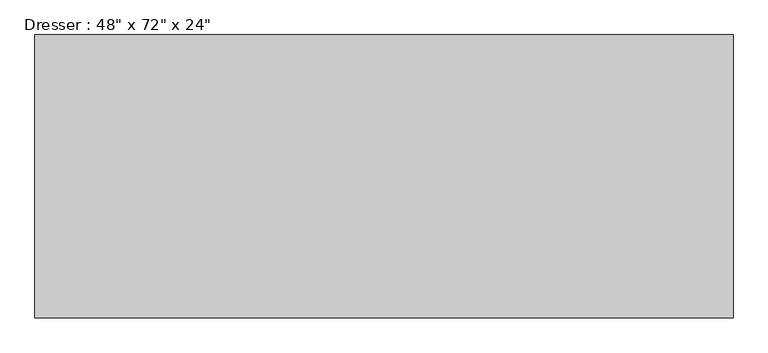
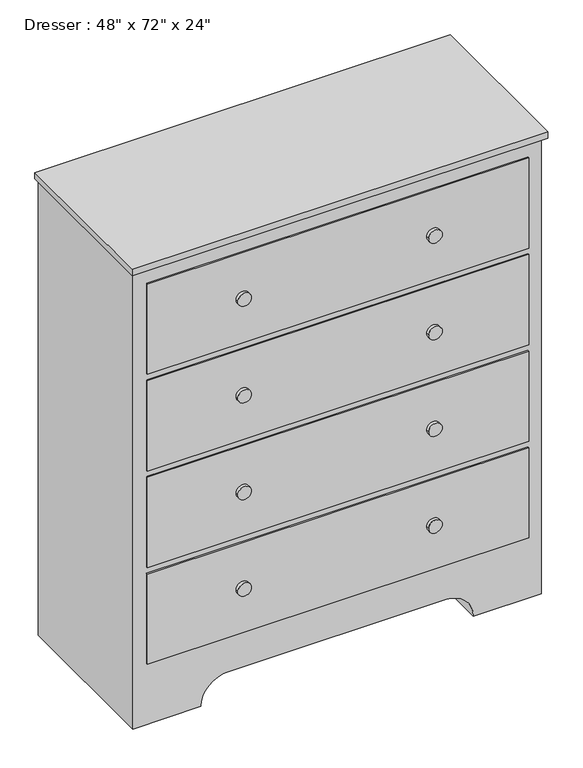
"""IFC4 building model written with IfcOpenShell, lengths in millimetres: furniture geometry."""

from ifc_helpers import new_model, si_unit, point, frame, frame_2d, origin, place, context, project, spatial, polyline, circle_curve, trimmed, segment, composite_curve, outline, extrude, source, transform, mapped, element, save


def furniture_d0678273(model_context):
    return source(origin(), model_context, "Body", "SweptSolid", [
        extrude(outline(polyline([(505.5067402, -58.3629541), (505.5067402, -687.0129541), (-1043.8932598, -687.0129541), (-1043.8932598, -58.3629541), (505.5067402, -58.3629541)])), frame((0.0, 0.0, 1803.4), z_axis=(0.0, 0.0, 1.0), x_axis=(1.0, 0.0, 0.0)), (0.0, 0.0, 1.0), 25.4),
        extrude(outline(composite_curve([segment(polyline([(0.0, 492.8067402), (1803.4, 492.8067402), (1803.4, -1031.1932598), (0.0, -1031.1932598), (0.0, -777.1932598)]), True, "CONTINUOUS"), segment(trimmed(circle_curve(frame_2d((0.0, -675.5932598)), 101.6), [point((0.0, -777.1932598))], [point((101.6, -675.5932598))], True, "CARTESIAN"), True, "CONTINUOUS"), segment(polyline([(101.6, -675.5932598), (101.6, 137.2067402)]), True, "CONTINUOUS"), segment(trimmed(circle_curve(frame_2d((0.0, 137.2067402)), 101.6), [point((101.6, 137.2067402))], [point((0.0, 238.8067402))], True, "CARTESIAN"), True, "CONTINUOUS"), segment(polyline([(0.0, 238.8067402), (0.0, 492.8067402)]), True, "CONTINUOUS")], self_intersect=False)), frame((0.0, -667.9629541, 0.0), z_axis=(0.0, 1.0, 0.0), x_axis=(0.0, 0.0, 1.0)), (0.0, 0.0, 1.0), 609.6),
        extrude(outline(composite_curve([segment(trimmed(circle_curve(frame_2d((1562.1, 86.4067402)), 25.4), [point((1562.1, 61.0067402))], [point((1562.1, 111.8067402))], False, "CARTESIAN"), True, "CONTINUOUS"), segment(trimmed(circle_curve(frame_2d((1562.1, 86.4067402)), 25.4), [point((1562.1, 111.8067402))], [point((1562.1, 61.0067402))], False, "CARTESIAN"), True, "CONTINUOUS")], self_intersect=False)), frame((0.0, -687.0129541, 0.0), z_axis=(0.0, 1.0, 0.0), x_axis=(0.0, 0.0, 1.0)), (0.0, 0.0, 1.0), 12.7),
        extrude(outline(composite_curve([segment(trimmed(circle_curve(frame_2d((1181.1, 86.4067402)), 25.4), [point((1181.1, 61.0067402))], [point((1181.1, 111.8067402))], False, "CARTESIAN"), True, "CONTINUOUS"), segment(trimmed(circle_curve(frame_2d((1181.1, 86.4067402)), 25.4), [point((1181.1, 111.8067402))], [point((1181.1, 61.0067402))], False, "CARTESIAN"), True, "CONTINUOUS")], self_intersect=False)), frame((0.0, -687.0129541, 0.0), z_axis=(0.0, 1.0, 0.0), x_axis=(0.0, 0.0, 1.0)), (0.0, 0.0, 1.0), 12.7),
        extrude(outline(composite_curve([segment(trimmed(circle_curve(frame_2d((800.1, 86.4067402)), 25.4), [point((800.1, 61.0067402))], [point((800.1, 111.8067402))], False, "CARTESIAN"), True, "CONTINUOUS"), segment(trimmed(circle_curve(frame_2d((800.1, 86.4067402)), 25.4), [point((800.1, 111.8067402))], [point((800.1, 61.0067402))], False, "CARTESIAN"), True, "CONTINUOUS")], self_intersect=False)), frame((0.0, -687.0129541, 0.0), z_axis=(0.0, 1.0, 0.0), x_axis=(0.0, 0.0, 1.0)), (0.0, 0.0, 1.0), 12.7),
        extrude(outline(composite_curve([segment(trimmed(circle_curve(frame_2d((419.1, 86.4067402)), 25.4), [point((419.1, 61.0067402))], [point((419.1, 111.8067402))], False, "CARTESIAN"), True, "CONTINUOUS"), segment(trimmed(circle_curve(frame_2d((419.1, 86.4067402)), 25.4), [point((419.1, 111.8067402))], [point((419.1, 61.0067402))], False, "CARTESIAN"), True, "CONTINUOUS")], self_intersect=False)), frame((0.0, -687.0129541, 0.0), z_axis=(0.0, 1.0, 0.0), x_axis=(0.0, 0.0, 1.0)), (0.0, 0.0, 1.0), 12.7),
        extrude(outline(composite_curve([segment(trimmed(circle_curve(frame_2d((419.1, -624.7932598)), 25.4), [point((419.1, -650.1932598))], [point((419.1, -599.3932598))], False, "CARTESIAN"), True, "CONTINUOUS"), segment(trimmed(circle_curve(frame_2d((419.1, -624.7932598)), 25.4), [point((419.1, -599.3932598))], [point((419.1, -650.1932598))], False, "CARTESIAN"), True, "CONTINUOUS")], self_intersect=False)), frame((0.0, -687.0129541, 0.0), z_axis=(0.0, 1.0, 0.0), x_axis=(0.0, 0.0, 1.0)), (0.0, 0.0, 1.0), 12.7),
        extrude(outline(composite_curve([segment(trimmed(circle_curve(frame_2d((800.1, -624.7932598)), 25.4), [point((800.1, -650.1932598))], [point((800.1, -599.3932598))], False, "CARTESIAN"), True, "CONTINUOUS"), segment(trimmed(circle_curve(frame_2d((800.1, -624.7932598)), 25.4), [point((800.1, -599.3932598))], [point((800.1, -650.1932598))], False, "CARTESIAN"), True, "CONTINUOUS")], self_intersect=False)), frame((0.0, -687.0129541, 0.0), z_axis=(0.0, 1.0, 0.0), x_axis=(0.0, 0.0, 1.0)), (0.0, 0.0, 1.0), 12.7),
        extrude(outline(composite_curve([segment(trimmed(circle_curve(frame_2d((1181.1, -624.7932598)), 25.4), [point((1181.1, -650.1932598))], [point((1181.1, -599.3932598))], False, "CARTESIAN"), True, "CONTINUOUS"), segment(trimmed(circle_curve(frame_2d((1181.1, -624.7932598)), 25.4), [point((1181.1, -599.3932598))], [point((1181.1, -650.1932598))], False, "CARTESIAN"), True, "CONTINUOUS")], self_intersect=False)), frame((0.0, -687.0129541, 0.0), z_axis=(0.0, 1.0, 0.0), x_axis=(0.0, 0.0, 1.0)), (0.0, 0.0, 1.0), 12.7),
        extrude(outline(composite_curve([segment(trimmed(circle_curve(frame_2d((1562.1, -624.7932598)), 25.4), [point((1562.1, -650.1932598))], [point((1562.1, -599.3932598))], False, "CARTESIAN"), True, "CONTINUOUS"), segment(trimmed(circle_curve(frame_2d((1562.1, -624.7932598)), 25.4), [point((1562.1, -599.3932598))], [point((1562.1, -650.1932598))], False, "CARTESIAN"), True, "CONTINUOUS")], self_intersect=False)), frame((0.0, -687.0129541, 0.0), z_axis=(0.0, 1.0, 0.0), x_axis=(0.0, 0.0, 1.0)), (0.0, 0.0, 1.0), 12.7),
        extrude(outline(polyline([(442.0067402, -674.3129541), (-980.3932598, -674.3129541), (-980.3932598, -667.9629541), (442.0067402, -667.9629541), (442.0067402, -674.3129541)])), frame((0.0, 0.0, 1384.3), z_axis=(0.0, 0.0, 1.0), x_axis=(1.0, 0.0, 0.0)), (0.0, 0.0, 1.0), 355.6),
        extrude(outline(polyline([(442.0067402, -674.3129541), (-980.3932598, -674.3129541), (-980.3932598, -667.9629541), (442.0067402, -667.9629541), (442.0067402, -674.3129541)])), frame((0.0, 0.0, 1003.3), z_axis=(0.0, 0.0, 1.0), x_axis=(1.0, 0.0, 0.0)), (0.0, 0.0, 1.0), 355.6),
        extrude(outline(polyline([(442.0067402, -674.3129541), (-980.3932598, -674.3129541), (-980.3932598, -667.9629541), (442.0067402, -667.9629541), (442.0067402, -674.3129541)])), frame((0.0, 0.0, 622.3), z_axis=(0.0, 0.0, 1.0), x_axis=(1.0, 0.0, 0.0)), (0.0, 0.0, 1.0), 355.6),
        extrude(outline(polyline([(442.0067402, -674.3129541), (-980.3932598, -674.3129541), (-980.3932598, -667.9629541), (442.0067402, -667.9629541), (442.0067402, -674.3129541)])), frame((0.0, 0.0, 241.3), z_axis=(0.0, 0.0, 1.0), x_axis=(1.0, 0.0, 0.0)), (0.0, 0.0, 1.0), 355.6),
    ])


if __name__ == "__main__":
    model = new_model("IFC4")
    model_context = context("Model", 3, world=origin())
    ifc_project = project(units=[si_unit("LENGTHUNIT", "METRE", prefix="MILLI")], contexts=[model_context])
    site = spatial("IfcSite", under=ifc_project)
    building = spatial("IfcBuilding", under=site)
    placement = place(None, origin())
    furniture_shape = furniture_d0678273(model_context)
    element("IfcFurniture", 1, ObjectType="Dresser : 48\" x 72\" x 24\"", at=placement, inside=building, context=model_context, shape_type="MappedRepresentation", body=[
        mapped(furniture_shape, transform((0.0, 0.0, 0.0), x_axis=(1.0, 0.0, 0.0), y_axis=(0.0, 1.0, 0.0), z_axis=(0.0, 0.0, 1.0))),
    ])
    save(model, "model.ifc")

# Revit data of these elements
# Type "Dresser : 48\" x 72\" x 24\""
#   Assembly Code = "E2020200"
#   Depth = 2' - 0"
#   Height = 6' - 0"
#   Width = 5' - 0"
#   Dresser Material = Laminate - Ivory, Glossy
#   Drawer Material = Laminate, Ivory, Matte
#   Knob Material = Cherry
#   Default Elevation = 0
# Element 1 (IfcFurniture, "Dresser : 48\" x 72\" x 24\"")
#   Materials on its faces: "Laminate, Ivory, Matte", "Cherry", "Laminate - Ivory, Glossy"
# Materials
#   "Laminate - Ivory, Glossy": colour RGB 247 247 239, transparency 0
#   "Laminate, Ivory, Matte": class "Plastic", colour RGB 247 247 239, transparency 0, Description = "Plastic Laminate - Ivory, Matte", Cost = 0
#   "Cherry": class "Wood", colour RGB 226 177 128, transparency 0, Description = "Prunus Serotina", Cost = 0
